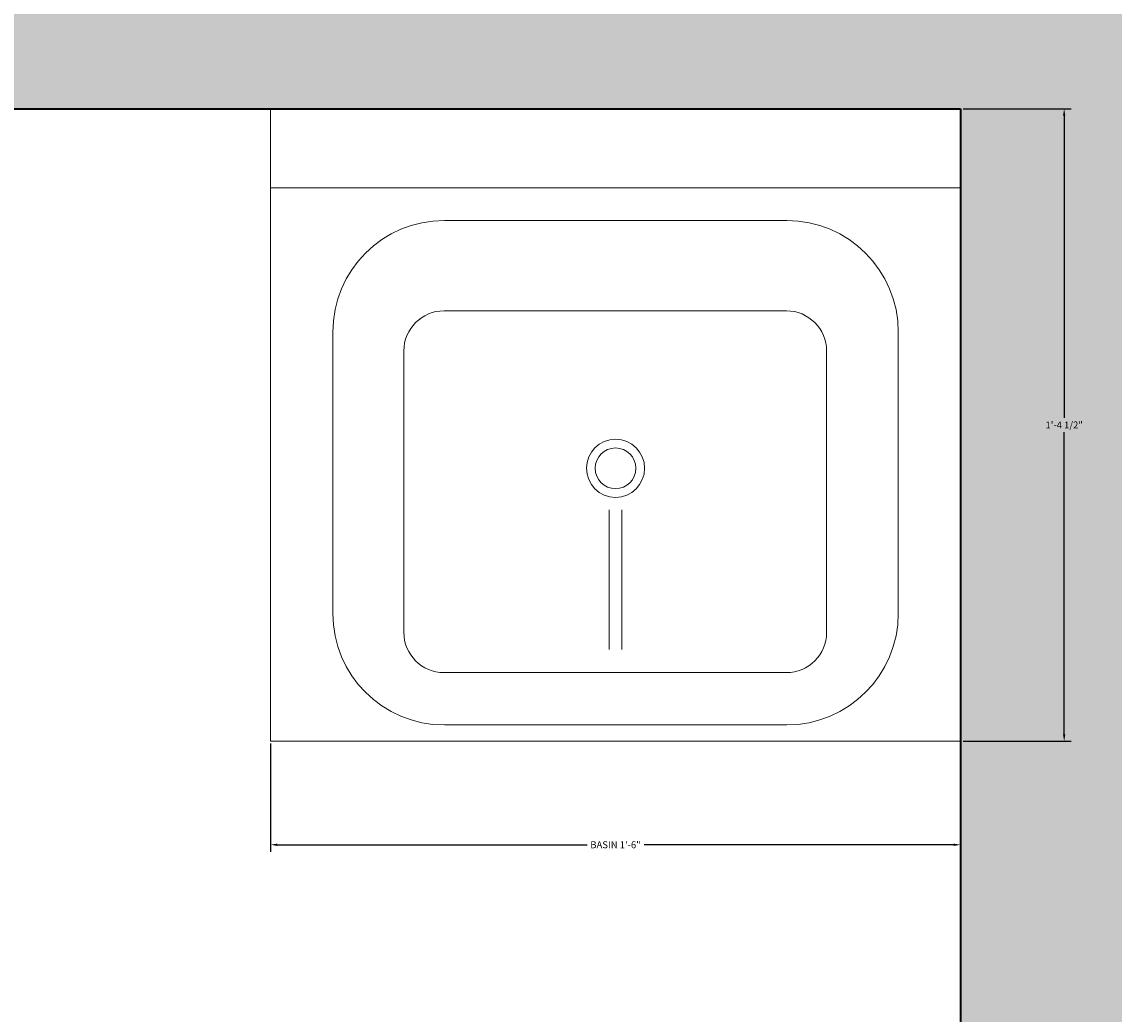
# Model space of a CAD drawing. Units: inches. Extents: x -9 to 505, y -680 to 48.
# Tile 14 of 17: x 96 to 124, y -139 to -114. Entities that reach past the tile are written whole.
import ezdxf

# ---------------------------------------------------------------- set-up
doc = ezdxf.new("R2010")
doc.units = ezdxf.units.IN
doc.header["$MEASUREMENT"] = 0
for name, color, linetype, lineweight in [('A-ANNO-DIMS', 2, 'Continuous', 18), ('A-FLOR-FIXT', 9, 'Continuous', 18), ('A-WALL', 7, 'Continuous', 35), ('A-WALL-PATT', 251, 'Continuous', 13)]:
    doc.layers.add(name, color=color, linetype=linetype, lineweight=lineweight)
doc.styles.get("Standard").update_dxf_attribs({"font": 'arial.ttf'})
doc.dimstyles.get("Standard").update_dxf_attribs({"dimtxt": 0.18, "dimasz": 0.18, "dimexe": 0.18, "dimexo": 0.0625, "dimgap": 0.09, "dimtad": 0, "dimtih": 1, "dimtoh": 1, "dimdec": 0, "dimzin": 0, "dimdsep": 46, "dimlunit": 3, "dimtxsty": 'Standard', "dimcen": 0.09, "dimadec": 0, "dimazin": 0, "dimtfac": 1, "dimtdec": 0, "dimtofl": 0, "dimtmove": 0, "dimatfit": 3, "dimfxl": 1, "dimtolj": 1, "dimtzin": 0, "dimarcsym": 0})

# ---------------------------------------------------------------- blocks, each defined once
blk = doc.blocks.new('М14 600х655')
for p, q in [((-655, 600), (-655, 0)), ((-655, 600), (-655, 0)), ((-655, 0), (-655, 600)), ((0, 600), (-655, 600)), ((0, 0), (0, 600)), ((0, 525), (-655, 525)), ((-165.1, 494.1), (-489.9, 494.1)), ((-165.4, 408.4), (-490.2, 408.4)), ((-595.8, 388.1), (-595.8, 121.3)), ((-59.2, 121.3), (-59.2, 388.1)), ((-528.4, 370.1), (-528.4, 103.3)), ((-127.2, 103.3), (-127.2, 370.1)), ((-333.5, 87.1), (-333.5, 219.6)), ((-321.5, 87.1), (-321.5, 219.6)), ((-490.2, 65.1), (-165.4, 65.1)), ((-489.9, 15.4), (-165.1, 15.4)), ((-655, 0), (-655, 0)), ((-655, 0), (-655, 0)), ((-655, 0), (0, 0)), ((-655, 0), (0, 0))]:
    blk.add_line(p, q)
for radius in [27.6, 19.3]:
    blk.add_circle((-327.5, 258.9), radius)
for centre, radius, start, end in [((-489.9, 388.1), 105.9, 90, 180), ((-165.1, 388.1), 105.9, 0, 90), ((-490.2, 370.1), 38.2, 90, 180), ((-165.4, 370.1), 38.2, 0, 90), ((-489.9, 121.3), 105.9, 180, 270), ((-165.1, 121.3), 105.9, 270, 0), ((-490.2, 103.3), 38.2, 180, 270), ((-165.4, 103.3), 38.2, 270, 0)]:
    blk.add_arc(centre, radius, start, end)
blk = doc.blocks.new('*D32')
at = {"layer": 'A-ANNO-DIMS', "color": 0, "lineweight": -2, "transparency": 16777216}
for p, q in [((102.391, -132.435), (102.391, -135.234)), ((120.264, -132.435), (120.264, -135.234)), ((102.571, -135.054), (110.59, -135.054)), ((120.084, -135.054), (112.065, -135.054))]:
    blk.add_line(p, q, dxfattribs=at)
at = {"layer": 'A-ANNO-DIMS', "color": 0, "transparency": 16777216}
for points in [[(102.571, -135.024), (102.571, -135.084), (102.391, -135.054)], [(120.084, -135.024), (120.084, -135.084), (120.264, -135.054)]]:
    blk.add_solid(points, dxfattribs=at)
at = {"layer": 'Defpoints', "color": 0, "transparency": 16777216}
for p in [(102.391, -132.373), (120.264, -132.373), (120.264, -135.054)]:
    blk.add_point(p, dxfattribs=at)
at = {"layer": 'A-ANNO-DIMS', "color": 0, "transparency": 16777216, "insert": (111.327, -135.054), "char_height": 0.18, "attachment_point": 5}
blk.add_mtext('\\A1;BASIN 1\'-6"', dxfattribs=at)
blk = doc.blocks.new('*D33')
at = {"layer": 'A-ANNO-DIMS', "color": 0, "lineweight": -2, "transparency": 16777216}
for p, q in [((120.326, -116.001), (123.124, -116.001)), ((122.944, -116.181), (122.944, -124.004)), ((122.944, -132.193), (122.944, -124.37)), ((120.326, -132.373), (123.124, -132.373))]:
    blk.add_line(p, q, dxfattribs=at)
at = {"layer": 'A-ANNO-DIMS', "color": 0, "transparency": 16777216}
for points in [[(122.914, -116.181), (122.974, -116.181), (122.944, -116.001)], [(122.914, -132.193), (122.974, -132.193), (122.944, -132.373)]]:
    blk.add_solid(points, dxfattribs=at)
at = {"layer": 'Defpoints', "color": 0, "transparency": 16777216}
for p in [(120.264, -116.001), (122.944, -116.001), (120.264, -132.373)]:
    blk.add_point(p, dxfattribs=at)
at = {"layer": 'A-ANNO-DIMS', "color": 0, "transparency": 16777216, "insert": (122.944, -124.187), "char_height": 0.18, "attachment_point": 5}
blk.add_mtext('\\A1;1\'-4 1/2"', dxfattribs=at)

msp = doc.modelspace()

# ---------------------------------------------------------------- hatches: boundary and pattern name
at = {"layer": 'A-WALL-PATT'}
h = msp.add_hatch(color=256, dxfattribs=at)
h.dxf.hatch_style = 1
h.paths.add_polyline_path([(101.641, 11.499), (48.264, 11.499), (48.264, 2.499), (72.264, 2.499), (72.264, -21.248), (81.264, -21.248), (81.264, 2.499), (101.641, 2.499)])
h.paths.add_polyline_path([(36.264, 2.499), (27.264, 2.499), (27.264, -6.918), (36.264, -6.918)])
h.paths.add_polyline_path([(81.264, -57.248), (72.264, -57.248), (72.264, -75.501), (81.264, -75.501)])
h.paths.add_polyline_path([(162.764, 11.499), (137.641, 11.499), (137.641, 2.499), (162.764, 2.499)])
h.paths.add_polyline_path([(179.264, 2.499), (174.764, 2.499), (174.764, -75.501), (179.264, -75.501), (179.264, -54.501), (229.514, -54.501), (229.514, -45.501), (179.264, -45.501)])
h.paths.add_polyline_path([(382.256, -45.501), (332.264, -45.501), (332.264, 2.499), (327.764, 2.499), (327.764, -45.501), (277.514, -45.501), (277.514, -54.501), (327.764, -54.501), (327.764, -111.501), (332.264, -111.501), (332.264, -54.501), (382.256, -54.501)])
h.paths.add_polyline_path([(332.264, -128.001), (327.764, -128.001), (327.764, -207.001), (332.264, -207.001)])
h.paths.add_polyline_path([(124.764, -111.501), (36.264, -111.501), (36.264, -116.001), (120.264, -116.001), (120.264, -168.501), (179.264, -168.501), (179.264, -164.001), (124.764, -164.001)])
h.paths.add_polyline_path([(96.264, -164.001), (36.264, -164.001), (36.264, -152.001), (27.264, -152.001), (27.264, -208.879), (36.264, -208.879), (36.264, -168.501), (96.264, -168.501)])
h.paths.add_polyline_path([(36.264, -244.879), (27.264, -244.879), (27.264, -287.001), (36.264, -287.001)])
h.paths.add_polyline_path([(179.264, -204.501), (174.764, -204.501), (174.764, -287.001), (179.264, -287.001)])
h.paths.add_polyline_path([(257.264, -296.001), (248.264, -296.001), (248.264, -446.001), (269.264, -446.001), (269.264, -437.001), (257.264, -437.001)])
h.paths.add_polyline_path([(90.264, -296.001), (81.264, -296.001), (81.264, -348.67), (90.264, -348.67)])
h.paths.add_polyline_path([(90.264, -384.67), (81.264, -384.67), (81.264, -416.001), (90.264, -416.001)])
h.paths.add_polyline_path([(170.264, -452.001), (36.264, -452.001), (36.264, -456.501), (165.764, -456.501), (165.764, -504.501), (165.133, -504.501), (165.133, -509.001), (170.264, -509.001)])
h.paths.add_polyline_path([(141.764, -504.501), (36.264, -504.501), (36.264, -492.501), (27.264, -492.501), (27.264, -565.959), (36.264, -565.959), (36.264, -509.001), (141.764, -509.001)])
h.paths.add_polyline_path([(36.264, -601.959), (27.264, -601.959), (27.264, -658.501), (36.264, -658.501)])
h.paths.add_polyline_path([(170.264, -670.501), (170.264, -634.501), (222.764, -634.501), (222.764, -625.501), (165.764, -625.501), (165.764, -670.501), (36.264, -670.501), (36.264, -679.501), (170.264, -679.501)])
h.paths.add_polyline_path([(332.264, -616.501), (433.894, -616.501), (433.894, -612.001), (332.264, -612.001), (332.264, -610.563), (327.764, -610.563), (327.764, -625.501), (270.764, -625.501), (270.764, -634.501), (327.764, -634.501), (327.764, -658.501), (332.264, -658.501)])
h.paths.add_polyline_path([(459.764, -670.501), (336.764, -670.501), (336.764, -679.501), (459.764, -679.501)])
h.paths.add_polyline_path([(468.764, -545.737), (459.764, -545.737), (459.764, -612.001), (457.894, -612.001), (457.894, -616.501), (459.764, -616.501), (459.764, -658.501), (468.764, -658.501)])
h.paths.add_polyline_path([(332.264, -446.001), (327.764, -446.001), (327.764, -574.563), (332.264, -574.563)])
h.paths.add_polyline_path([(327.764, -437.001), (305.264, -437.001), (305.264, -446.001), (327.764, -446.001)])
h.paths.add_polyline_path([(459.764, -437.001), (348.764, -437.001), (348.764, -446.001), (459.764, -446.001)])
h.paths.add_polyline_path([(468.764, -458.001), (459.764, -458.001), (459.764, -509.737), (468.764, -509.737)])
h.paths.add_polyline_path([(468.764, -365.001), (459.764, -365.001), (459.764, -437.001), (468.764, -437.001)])
h.paths.add_polyline_path([(468.764, -299.601), (459.764, -299.601), (459.764, -344.001), (468.764, -344.001)])
h.paths.add_polyline_path([(468.764, -184.739), (459.764, -184.739), (459.764, -231.001), (401.264, -231.001), (401.264, -235.501), (459.764, -235.501), (459.764, -275.601), (468.764, -275.601)])
h.paths.add_polyline_path([(390.764, -356.001), (342.764, -356.001), (342.764, -365.001), (390.764, -365.001)])
h.paths.add_polyline_path([(459.764, -356.001), (405.764, -356.001), (405.764, -365.001), (459.764, -365.001)])
h.paths.add_polyline_path([(405.764, -296.001), (396.764, -296.001), (396.764, -356.001), (405.764, -356.001)])
h.paths.add_polyline_path([(336.764, -296.001), (327.764, -296.001), (327.764, -356.001), (336.764, -356.001)])
h.paths.add_polyline_path([(468.764, -9.501), (459.764, -9.501), (459.764, -45.501), (418.256, -45.501), (418.256, -54.501), (468.764, -54.501)])
h.paths.add_polyline_path([(468.764, -54.501), (459.764, -54.501), (459.764, -111.501), (468.764, -111.501)])
h.paths.add_polyline_path([(468.764, -128.001), (459.764, -128.001), (459.764, -148.739), (468.764, -148.739)])

# ---------------------------------------------------------------- linework, layer by layer
at = {"layer": 'A-WALL'}
for p, q in [((36.264, -116.001), (120.264, -116.001)), ((120.264, -116.001), (120.264, -168.501))]:
    msp.add_line(p, q, dxfattribs=at)

# ---------------------------------------------------------------- block references
at = {"layer": 'A-FLOR-FIXT', "xscale": 0.0272863039339927, "yscale": 0.0272863039339927, "zscale": 0.0272863039339927}
msp.add_blockref('М14 600х655', (120.264, -132.373), dxfattribs=at)

# ---------------------------------------------------------------- dimensions: what is measured, and where the dimension line sits
at = {"layer": 'A-ANNO-DIMS'}
dim = msp.add_linear_dim(base=(122.944, -116.001), p1=(120.264, -132.373), p2=(120.264, -116.001), angle=90, dimstyle='Standard', override={"dimdec": 1, "dimlfac": 1, "dimrnd": 0, "dimzin": 1, "dimdsep": 46, "dimlunit": 4, "dimfrac": 2}, dxfattribs=at)
dim.commit()
dim.dimension.update_dxf_attribs({"geometry": '*D33', "text_midpoint": (122.944, -124.187)})
dim = msp.add_linear_dim(base=(120.264, -135.054), p1=(102.391, -132.373), p2=(120.264, -132.373), text='BASIN <>', dimstyle='Standard', override={"dimdec": 1, "dimlfac": 1, "dimrnd": 0, "dimzin": 1, "dimdsep": 46, "dimlunit": 4, "dimfrac": 2}, dxfattribs=at)
dim.commit()
dim.dimension.update_dxf_attribs({"geometry": '*D32', "text_midpoint": (111.327, -135.054)})

doc.saveas('drawing.dxf')
